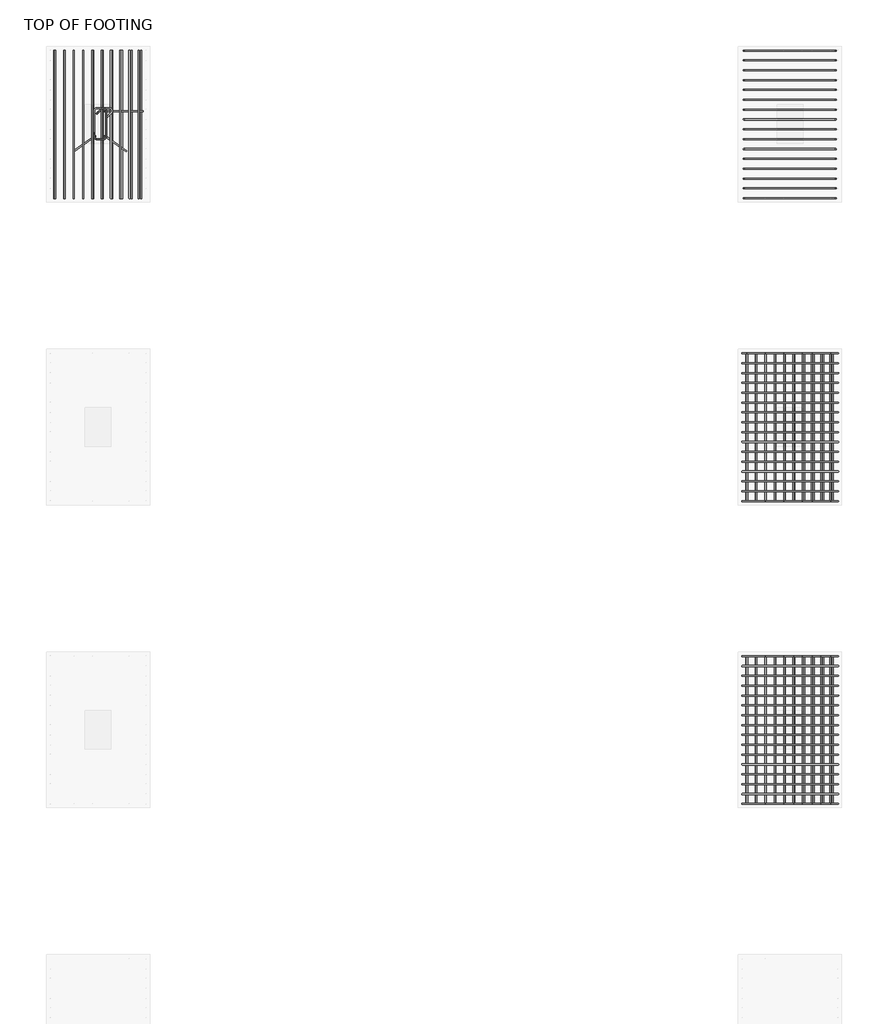
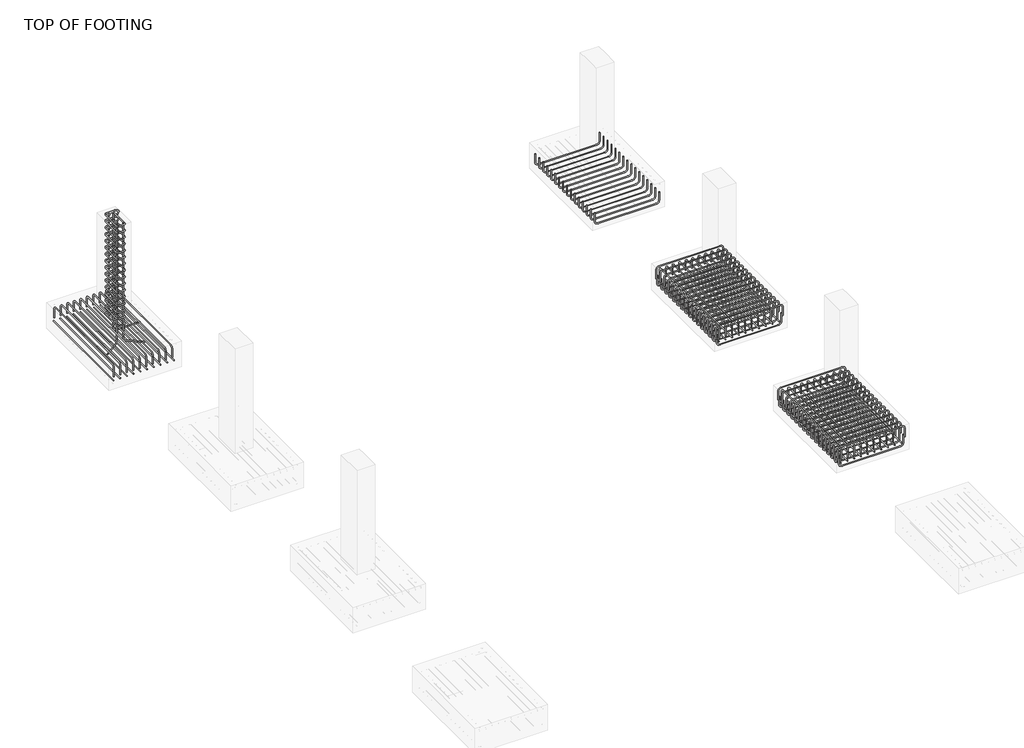
# One storey, part 4 of 8: 15 reinforcing bars.
"""IFC4 building model written with IfcOpenShell, lengths in millimetres."""

from ifc_helpers import new_model, si_unit, point, frame, origin, place, context, project, spatial, polyline, circle_curve, trimmed, segment, composite_curve, source, transform, mapped, element, save
from ifc_brep_helpers import swept_disk

model = new_model("IFC4")

# Units and contexts
model_context = context("Model", 3, world=origin())
ifc_project = project(units=[si_unit("LENGTHUNIT", "METRE", prefix="MILLI")], contexts=[model_context])

# Site, building, storey
site = spatial("IfcSite", under=ifc_project)
building = spatial("IfcBuilding", under=site)
storey = spatial("IfcBuildingStorey", under=building, Name="TOP OF FOOTING", Elevation=-1828.8)

# Reinforcing bars
placement = place(None, origin())
reinforcing_bar_shape = source(origin(), model_context, "Body", "SolidModel", [
    swept_disk(composite_curve([segment(polyline([(-12339.592709, 16632.7008557, -2155.1176129), (-12339.592709, 14912.7008557, -2155.1176129)]), True, "CONTINUOUS")], self_intersect=False), 6.35),
])
element("IfcReinforcingBar", 1, at=placement, inside=storey, context=model_context, shape_type="MappedRepresentation", body=[
    mapped(reinforcing_bar_shape, transform((0.0, 0.0, 0.0), x_axis=(1.0, 0.0, 0.0), y_axis=(0.0, 1.0, 0.0), z_axis=(0.0, 0.0, 1.0))),
    mapped(reinforcing_bar_shape, transform((111.602188, 0.0, 0.0), x_axis=(1.0, 0.0, 0.0), y_axis=(0.0, 1.0, 0.0), z_axis=(0.0, 0.0, 1.0))),
    mapped(reinforcing_bar_shape, transform((223.2043759, 0.0, 0.0), x_axis=(1.0, 0.0, 0.0), y_axis=(0.0, 1.0, 0.0), z_axis=(0.0, 0.0, 1.0))),
    mapped(reinforcing_bar_shape, transform((334.8065639, 0.0, 0.0), x_axis=(1.0, 0.0, 0.0), y_axis=(0.0, 1.0, 0.0), z_axis=(0.0, 0.0, 1.0))),
    mapped(reinforcing_bar_shape, transform((446.4087519, 0.0, 0.0), x_axis=(1.0, 0.0, 0.0), y_axis=(0.0, 1.0, 0.0), z_axis=(0.0, 0.0, 1.0))),
    mapped(reinforcing_bar_shape, transform((558.0109398, 0.0, 0.0), x_axis=(1.0, 0.0, 0.0), y_axis=(0.0, 1.0, 0.0), z_axis=(0.0, 0.0, 1.0))),
    mapped(reinforcing_bar_shape, transform((669.6131278, 0.0, 0.0), x_axis=(1.0, 0.0, 0.0), y_axis=(0.0, 1.0, 0.0), z_axis=(0.0, 0.0, 1.0))),
    mapped(reinforcing_bar_shape, transform((781.2153158, 0.0, 0.0), x_axis=(1.0, 0.0, 0.0), y_axis=(0.0, 1.0, 0.0), z_axis=(0.0, 0.0, 1.0))),
    mapped(reinforcing_bar_shape, transform((892.8175037, 0.0, 0.0), x_axis=(1.0, 0.0, 0.0), y_axis=(0.0, 1.0, 0.0), z_axis=(0.0, 0.0, 1.0))),
    mapped(reinforcing_bar_shape, transform((1004.4196917, 0.0, 0.0), x_axis=(1.0, 0.0, 0.0), y_axis=(0.0, 1.0, 0.0), z_axis=(0.0, 0.0, 1.0))),
])
reinforcing_bar_2_shape = source(origin(), model_context, "Body", "SolidModel", [
    swept_disk(composite_curve([segment(polyline([(-11364.2651981, 16626.3508557, -2094.6521303), (-11364.2651981, 16626.3508557, -1947.3521303)]), True, "CONTINUOUS"), segment(trimmed(circle_curve(frame((-11364.2651981, 16580.0008557, -1947.3521303), z_axis=(1.0, 0.0, 0.0), x_axis=(0.0, 46.349999999998545, 0.0)), 46.35), [point((-11364.2651981, 16626.3508557, -1947.3521303))], [point((-11364.2651981, 16580.0008557, -1901.0021303))], True, "CARTESIAN"), True, "CONTINUOUS"), segment(polyline([(-11364.2651981, 16580.0008557, -1901.0021303), (-11364.2651981, 14965.4008557, -1901.0021303)]), True, "CONTINUOUS"), segment(trimmed(circle_curve(frame((-11364.2651981, 14965.4008557, -1947.3521303), z_axis=(1.0, 0.0, 0.0), x_axis=(0.0, 0.0, 46.34999999999991)), 46.35), [point((-11364.2651981, 14965.4008557, -1901.0021303))], [point((-11364.2651981, 14919.0508557, -1947.3521303))], True, "CARTESIAN"), True, "CONTINUOUS"), segment(polyline([(-11364.2651981, 14919.0508557, -1947.3521303), (-11364.2651981, 14919.0508557, -2094.6521303)]), True, "CONTINUOUS")], self_intersect=False), 6.35),
])
element("IfcReinforcingBar", 2, at=placement, inside=storey, context=model_context, shape_type="MappedRepresentation", body=[
    mapped(reinforcing_bar_2_shape, transform((0.0, 0.0, 0.0), x_axis=(1.0, 0.0, 0.0), y_axis=(0.0, 1.0, 0.0), z_axis=(0.0, 0.0, 1.0))),
    mapped(reinforcing_bar_2_shape, transform((-107.1680233, 0.0, 0.0), x_axis=(1.0, 0.0, 0.0), y_axis=(0.0, 1.0, 0.0), z_axis=(0.0, 0.0, 1.0))),
    mapped(reinforcing_bar_2_shape, transform((-214.3360466, 0.0, 0.0), x_axis=(1.0, 0.0, 0.0), y_axis=(0.0, 1.0, 0.0), z_axis=(0.0, 0.0, 1.0))),
    mapped(reinforcing_bar_2_shape, transform((-321.5040699, 0.0, 0.0), x_axis=(1.0, 0.0, 0.0), y_axis=(0.0, 1.0, 0.0), z_axis=(0.0, 0.0, 1.0))),
    mapped(reinforcing_bar_2_shape, transform((-428.6720932, 0.0, 0.0), x_axis=(1.0, 0.0, 0.0), y_axis=(0.0, 1.0, 0.0), z_axis=(0.0, 0.0, 1.0))),
    mapped(reinforcing_bar_2_shape, transform((-535.8401165, 0.0, 0.0), x_axis=(1.0, 0.0, 0.0), y_axis=(0.0, 1.0, 0.0), z_axis=(0.0, 0.0, 1.0))),
    mapped(reinforcing_bar_2_shape, transform((-643.0081398, 0.0, 0.0), x_axis=(1.0, 0.0, 0.0), y_axis=(0.0, 1.0, 0.0), z_axis=(0.0, 0.0, 1.0))),
    mapped(reinforcing_bar_2_shape, transform((-750.176163, 0.0, 0.0), x_axis=(1.0, 0.0, 0.0), y_axis=(0.0, 1.0, 0.0), z_axis=(0.0, 0.0, 1.0))),
    mapped(reinforcing_bar_2_shape, transform((-857.3441863, 0.0, 0.0), x_axis=(1.0, 0.0, 0.0), y_axis=(0.0, 1.0, 0.0), z_axis=(0.0, 0.0, 1.0))),
    mapped(reinforcing_bar_2_shape, transform((-964.5122096, 0.0, 0.0), x_axis=(1.0, 0.0, 0.0), y_axis=(0.0, 1.0, 0.0), z_axis=(0.0, 0.0, 1.0))),
])
reinforcing_bar_3_shape = source(origin(), model_context, "Body", "SolidModel", [
    swept_disk(composite_curve([segment(polyline([(-11851.3503281, 15894.7413561, -46.35), (-11795.6067652, 15950.484919, -46.35)]), True, "CONTINUOUS"), segment(trimmed(circle_curve(frame((-11773.4389676, 15928.3171214, -46.35), z_axis=(0.0, 0.0, -1.0), x_axis=(-22.167797600000995, 22.167797600000995, 0.0)), 31.35), [point((-11795.6067652, 15950.484919, -46.35))], [point((-11742.0889676, 15928.3171214, -46.35))], True, "CARTESIAN"), True, "CONTINUOUS"), segment(polyline([(-11742.0889676, 15928.3171214, -46.35), (-11742.0889676, 15633.7171214, -46.35)]), True, "CONTINUOUS"), segment(trimmed(circle_curve(frame((-11773.4389676, 15633.7171214, -46.35), z_axis=(0.0, 0.0, -1.0), x_axis=(31.349999999998545, 0.0, 0.0)), 31.35), [point((-11742.0889676, 15633.7171214, -46.35))], [point((-11773.4389676, 15602.3671214, -46.35))], True, "CARTESIAN"), True, "CONTINUOUS"), segment(polyline([(-11773.4389676, 15602.3671214, -46.35), (-11848.385177, 15602.3671214, -46.35)]), True, "CONTINUOUS"), segment(trimmed(circle_curve(frame((-11848.385177, 15633.6973363, -45.2363875), z_axis=(0.0, 0.035521928334481916, -0.9993688971583016), x_axis=(0.0, -31.33021489999919, -1.1136125000000021)), 31.35), [point((-11848.385177, 15602.3671214, -46.35))], [point((-11879.735177, 15633.6973363, -45.2363875))], True, "CARTESIAN"), True, "CONTINUOUS"), segment(polyline([(-11879.735177, 15633.6973363, -45.2363875), (-11879.735177, 15928.3369065, -34.7636125)]), True, "CONTINUOUS"), segment(trimmed(circle_curve(frame((-11848.385177, 15928.3369065, -34.7636125), z_axis=(0.0, 0.035521928334481916, -0.9993688971583016), x_axis=(-31.350000000000364, 0.0, 0.0)), 31.35), [point((-11879.735177, 15928.3369065, -34.7636125))], [point((-11848.385177, 15959.6671214, -33.65))], True, "CARTESIAN"), True, "CONTINUOUS"), segment(polyline([(-11848.385177, 15959.6671214, -33.65), (-11703.785177, 15959.6671214, -33.65)]), True, "CONTINUOUS"), segment(trimmed(circle_curve(frame((-11703.785177, 15928.3171214, -33.65), z_axis=(0.0, 0.0, -1.0), x_axis=(0.0, 31.350000000000364, 0.0)), 31.35), [point((-11703.785177, 15959.6671214, -33.65))], [point((-11681.6173794, 15906.1493238, -33.65))], True, "CARTESIAN"), True, "CONTINUOUS"), segment(polyline([(-11681.6173794, 15906.1493238, -33.65), (-11737.3609424, 15850.4057609, -33.65)]), True, "CONTINUOUS")], self_intersect=False), 6.35),
])
element("IfcReinforcingBar", 3, at=placement, inside=storey, context=model_context, shape_type="MappedRepresentation", body=[
    mapped(reinforcing_bar_3_shape, transform((0.0, 0.0, 0.0), x_axis=(1.0, 0.0, 0.0), y_axis=(0.0, 1.0, 0.0), z_axis=(0.0, 0.0, 1.0))),
    mapped(reinforcing_bar_3_shape, transform((0.0, 0.0, -115.74), x_axis=(1.0, 0.0, 0.0), y_axis=(0.0, 1.0, 0.0), z_axis=(0.0, 0.0, 1.0))),
    mapped(reinforcing_bar_3_shape, transform((0.0, 0.0, -231.48), x_axis=(1.0, 0.0, 0.0), y_axis=(0.0, 1.0, 0.0), z_axis=(0.0, 0.0, 1.0))),
    mapped(reinforcing_bar_3_shape, transform((0.0, 0.0, -347.22), x_axis=(1.0, 0.0, 0.0), y_axis=(0.0, 1.0, 0.0), z_axis=(0.0, 0.0, 1.0))),
    mapped(reinforcing_bar_3_shape, transform((0.0, 0.0, -462.96), x_axis=(1.0, 0.0, 0.0), y_axis=(0.0, 1.0, 0.0), z_axis=(0.0, 0.0, 1.0))),
    mapped(reinforcing_bar_3_shape, transform((0.0, 0.0, -578.7), x_axis=(1.0, 0.0, 0.0), y_axis=(0.0, 1.0, 0.0), z_axis=(0.0, 0.0, 1.0))),
    mapped(reinforcing_bar_3_shape, transform((0.0, 0.0, -694.44), x_axis=(1.0, 0.0, 0.0), y_axis=(0.0, 1.0, 0.0), z_axis=(0.0, 0.0, 1.0))),
    mapped(reinforcing_bar_3_shape, transform((0.0, 0.0, -810.18), x_axis=(1.0, 0.0, 0.0), y_axis=(0.0, 1.0, 0.0), z_axis=(0.0, 0.0, 1.0))),
    mapped(reinforcing_bar_3_shape, transform((0.0, 0.0, -925.92), x_axis=(1.0, 0.0, 0.0), y_axis=(0.0, 1.0, 0.0), z_axis=(0.0, 0.0, 1.0))),
    mapped(reinforcing_bar_3_shape, transform((0.0, 0.0, -1041.66), x_axis=(1.0, 0.0, 0.0), y_axis=(0.0, 1.0, 0.0), z_axis=(0.0, 0.0, 1.0))),
    mapped(reinforcing_bar_3_shape, transform((0.0, 0.0, -1157.4), x_axis=(1.0, 0.0, 0.0), y_axis=(0.0, 1.0, 0.0), z_axis=(0.0, 0.0, 1.0))),
    mapped(reinforcing_bar_3_shape, transform((0.0, 0.0, -1273.14), x_axis=(1.0, 0.0, 0.0), y_axis=(0.0, 1.0, 0.0), z_axis=(0.0, 0.0, 1.0))),
    mapped(reinforcing_bar_3_shape, transform((0.0, 0.0, -1388.88), x_axis=(1.0, 0.0, 0.0), y_axis=(0.0, 1.0, 0.0), z_axis=(0.0, 0.0, 1.0))),
    mapped(reinforcing_bar_3_shape, transform((0.0, 0.0, -1504.62), x_axis=(1.0, 0.0, 0.0), y_axis=(0.0, 1.0, 0.0), z_axis=(0.0, 0.0, 1.0))),
    mapped(reinforcing_bar_3_shape, transform((0.0, 0.0, -1620.36), x_axis=(1.0, 0.0, 0.0), y_axis=(0.0, 1.0, 0.0), z_axis=(0.0, 0.0, 1.0))),
    mapped(reinforcing_bar_3_shape, transform((0.0, 0.0, -1736.1), x_axis=(1.0, 0.0, 0.0), y_axis=(0.0, 1.0, 0.0), z_axis=(0.0, 0.0, 1.0))),
])
element("IfcReinforcingBar", 4, at=placement, inside=storey, context=model_context, shape_type="SolidModel", body=[
    swept_disk(composite_curve([segment(polyline([(-11755.8874017, 15924.2508557, -40.0), (-11755.8874017, 15924.2508557, -2055.5685723)]), True, "CONTINUOUS"), segment(trimmed(circle_curve(frame((-11709.5374017, 15924.2508557, -2055.5685723), z_axis=(0.0, -1.0, 0.0), x_axis=(-46.350000000000364, 0.0, 0.0)), 46.35), [point((-11755.8874017, 15924.2508557, -2055.5685723))], [point((-11709.5374017, 15924.2508557, -2101.9185723))], True, "CARTESIAN"), True, "CONTINUOUS"), segment(polyline([(-11709.5374017, 15924.2508557, -2101.9185723), (-11315.6661764, 15924.2508557, -2101.9185723)]), True, "CONTINUOUS")], self_intersect=False), 6.35),
])
element("IfcReinforcingBar", 5, at=placement, inside=storey, context=model_context, shape_type="SolidModel", body=[
    swept_disk(composite_curve([segment(polyline([(-11755.8874017, 15637.7833871, -40.0), (-11755.8874017, 15637.7833871, -2055.5685723)]), True, "CONTINUOUS"), segment(trimmed(circle_curve(frame((-11717.9197045, 15611.1981193, -2055.5685723), z_axis=(-0.5735764363510459, -0.819152044288992, 0.0), x_axis=(-37.96769719999975, 26.58526780000102, 0.0)), 46.35), [point((-11755.8874017, 15637.7833871, -2055.5685723))], [point((-11717.9197045, 15611.1981193, -2101.9185723))], True, "CARTESIAN"), True, "CONTINUOUS"), segment(polyline([(-11717.9197045, 15611.1981193, -2101.9185723), (-11506.0932621, 15462.8756476, -2101.9185723)]), True, "CONTINUOUS")], self_intersect=False), 6.35),
])
element("IfcReinforcingBar", 6, at=placement, inside=storey, context=model_context, shape_type="SolidModel", body=[
    swept_disk(composite_curve([segment(polyline([(-11865.9367429, 15637.7833871, -40.0), (-11865.9367429, 15637.7833871, -2055.5685723)]), True, "CONTINUOUS"), segment(trimmed(circle_curve(frame((-11903.9044402, 15611.1981193, -2055.5685723), z_axis=(-0.5735764363510459, 0.819152044288992, 0.0), x_axis=(37.96769730000051, 26.58526780000102, 0.0)), 46.35), [point((-11865.9367429, 15637.7833871, -2055.5685723))], [point((-11903.9044402, 15611.1981193, -2101.9185723))], True, "CARTESIAN"), True, "CONTINUOUS"), segment(polyline([(-11903.9044402, 15611.1981193, -2101.9185723), (-12115.7308826, 15462.8756476, -2101.9185723)]), True, "CONTINUOUS")], self_intersect=False), 6.35),
])
reinforcing_bar_4_shape = source(origin(), model_context, "Body", "SolidModel", [
    swept_disk(composite_curve([segment(polyline([(-3301.5220197, 16626.3508557, -2021.4413313), (-3301.5220197, 16626.3508557, -2168.7413313)]), True, "CONTINUOUS"), segment(trimmed(circle_curve(frame((-3347.8720197, 16626.3508557, -2168.7413313), z_axis=(0.0, 1.0, 0.0), x_axis=(46.34999999999991, 0.0, 0.0)), 46.35), [point((-3301.5220197, 16626.3508557, -2168.7413313))], [point((-3347.8720197, 16626.3508557, -2215.0913313))], True, "CARTESIAN"), True, "CONTINUOUS"), segment(polyline([(-3347.8720197, 16626.3508557, -2215.0913313), (-4320.167031, 16626.3508557, -2215.0913313)]), True, "CONTINUOUS"), segment(trimmed(circle_curve(frame((-4320.167031, 16626.3508557, -2168.7413313), z_axis=(0.0, 1.0, 0.0), x_axis=(0.0, 0.0, -46.34999999999991)), 46.35), [point((-4320.167031, 16626.3508557, -2215.0913313))], [point((-4366.517031, 16626.3508557, -2168.7413313))], True, "CARTESIAN"), True, "CONTINUOUS"), segment(polyline([(-4366.517031, 16626.3508557, -2168.7413313), (-4366.517031, 16626.3508557, -2021.4413313)]), True, "CONTINUOUS")], self_intersect=False), 6.35),
])
element("IfcReinforcingBar", 7, at=placement, inside=storey, context=model_context, shape_type="MappedRepresentation", body=[
    mapped(reinforcing_bar_4_shape, transform((0.0, 0.0, 0.0), x_axis=(1.0, 0.0, 0.0), y_axis=(0.0, 1.0, 0.0), z_axis=(0.0, 0.0, 1.0))),
    mapped(reinforcing_bar_4_shape, transform((0.0, -113.82, 0.0), x_axis=(1.0, 0.0, 0.0), y_axis=(0.0, 1.0, 0.0), z_axis=(0.0, 0.0, 1.0))),
    mapped(reinforcing_bar_4_shape, transform((0.0, -227.64, 0.0), x_axis=(1.0, 0.0, 0.0), y_axis=(0.0, 1.0, 0.0), z_axis=(0.0, 0.0, 1.0))),
    mapped(reinforcing_bar_4_shape, transform((0.0, -341.46, 0.0), x_axis=(1.0, 0.0, 0.0), y_axis=(0.0, 1.0, 0.0), z_axis=(0.0, 0.0, 1.0))),
    mapped(reinforcing_bar_4_shape, transform((0.0, -455.28, 0.0), x_axis=(1.0, 0.0, 0.0), y_axis=(0.0, 1.0, 0.0), z_axis=(0.0, 0.0, 1.0))),
    mapped(reinforcing_bar_4_shape, transform((0.0, -569.1, 0.0), x_axis=(1.0, 0.0, 0.0), y_axis=(0.0, 1.0, 0.0), z_axis=(0.0, 0.0, 1.0))),
    mapped(reinforcing_bar_4_shape, transform((0.0, -682.92, 0.0), x_axis=(1.0, 0.0, 0.0), y_axis=(0.0, 1.0, 0.0), z_axis=(0.0, 0.0, 1.0))),
    mapped(reinforcing_bar_4_shape, transform((0.0, -796.74, 0.0), x_axis=(1.0, 0.0, 0.0), y_axis=(0.0, 1.0, 0.0), z_axis=(0.0, 0.0, 1.0))),
    mapped(reinforcing_bar_4_shape, transform((0.0, -910.56, 0.0), x_axis=(1.0, 0.0, 0.0), y_axis=(0.0, 1.0, 0.0), z_axis=(0.0, 0.0, 1.0))),
    mapped(reinforcing_bar_4_shape, transform((0.0, -1024.38, 0.0), x_axis=(1.0, 0.0, 0.0), y_axis=(0.0, 1.0, 0.0), z_axis=(0.0, 0.0, 1.0))),
    mapped(reinforcing_bar_4_shape, transform((0.0, -1138.2, 0.0), x_axis=(1.0, 0.0, 0.0), y_axis=(0.0, 1.0, 0.0), z_axis=(0.0, 0.0, 1.0))),
    mapped(reinforcing_bar_4_shape, transform((0.0, -1252.02, 0.0), x_axis=(1.0, 0.0, 0.0), y_axis=(0.0, 1.0, 0.0), z_axis=(0.0, 0.0, 1.0))),
    mapped(reinforcing_bar_4_shape, transform((0.0, -1365.84, 0.0), x_axis=(1.0, 0.0, 0.0), y_axis=(0.0, 1.0, 0.0), z_axis=(0.0, 0.0, 1.0))),
    mapped(reinforcing_bar_4_shape, transform((0.0, -1479.66, 0.0), x_axis=(1.0, 0.0, 0.0), y_axis=(0.0, 1.0, 0.0), z_axis=(0.0, 0.0, 1.0))),
    mapped(reinforcing_bar_4_shape, transform((0.0, -1593.48, 0.0), x_axis=(1.0, 0.0, 0.0), y_axis=(0.0, 1.0, 0.0), z_axis=(0.0, 0.0, 1.0))),
    mapped(reinforcing_bar_4_shape, transform((0.0, -1707.3, 0.0), x_axis=(1.0, 0.0, 0.0), y_axis=(0.0, 1.0, 0.0), z_axis=(0.0, 0.0, 1.0))),
])
reinforcing_bar_5_shape = source(origin(), model_context, "Body", "SolidModel", [
    swept_disk(composite_curve([segment(polyline([(-3301.5220197, 13126.3508557, -2021.4413313), (-3301.5220197, 13126.3508557, -2168.7413313)]), True, "CONTINUOUS"), segment(trimmed(circle_curve(frame((-3347.8720197, 13126.3508557, -2168.7413313), z_axis=(0.0, 1.0, 0.0), x_axis=(46.34999999999991, 0.0, 0.0)), 46.35), [point((-3301.5220197, 13126.3508557, -2168.7413313))], [point((-3347.8720197, 13126.3508557, -2215.0913313))], True, "CARTESIAN"), True, "CONTINUOUS"), segment(polyline([(-3347.8720197, 13126.3508557, -2215.0913313), (-4320.167031, 13126.3508557, -2215.0913313)]), True, "CONTINUOUS"), segment(trimmed(circle_curve(frame((-4320.167031, 13126.3508557, -2168.7413313), z_axis=(0.0, 1.0, 0.0), x_axis=(0.0, 0.0, -46.34999999999991)), 46.35), [point((-4320.167031, 13126.3508557, -2215.0913313))], [point((-4366.517031, 13126.3508557, -2168.7413313))], True, "CARTESIAN"), True, "CONTINUOUS"), segment(polyline([(-4366.517031, 13126.3508557, -2168.7413313), (-4366.517031, 13126.3508557, -2021.4413313)]), True, "CONTINUOUS")], self_intersect=False), 6.35),
])
element("IfcReinforcingBar", 8, at=placement, inside=storey, context=model_context, shape_type="MappedRepresentation", body=[
    mapped(reinforcing_bar_5_shape, transform((0.0, 0.0, 0.0), x_axis=(1.0, 0.0, 0.0), y_axis=(0.0, 1.0, 0.0), z_axis=(0.0, 0.0, 1.0))),
    mapped(reinforcing_bar_5_shape, transform((0.0, -113.82, 0.0), x_axis=(1.0, 0.0, 0.0), y_axis=(0.0, 1.0, 0.0), z_axis=(0.0, 0.0, 1.0))),
    mapped(reinforcing_bar_5_shape, transform((0.0, -227.64, 0.0), x_axis=(1.0, 0.0, 0.0), y_axis=(0.0, 1.0, 0.0), z_axis=(0.0, 0.0, 1.0))),
    mapped(reinforcing_bar_5_shape, transform((0.0, -341.46, 0.0), x_axis=(1.0, 0.0, 0.0), y_axis=(0.0, 1.0, 0.0), z_axis=(0.0, 0.0, 1.0))),
    mapped(reinforcing_bar_5_shape, transform((0.0, -455.28, 0.0), x_axis=(1.0, 0.0, 0.0), y_axis=(0.0, 1.0, 0.0), z_axis=(0.0, 0.0, 1.0))),
    mapped(reinforcing_bar_5_shape, transform((0.0, -569.1, 0.0), x_axis=(1.0, 0.0, 0.0), y_axis=(0.0, 1.0, 0.0), z_axis=(0.0, 0.0, 1.0))),
    mapped(reinforcing_bar_5_shape, transform((0.0, -682.92, 0.0), x_axis=(1.0, 0.0, 0.0), y_axis=(0.0, 1.0, 0.0), z_axis=(0.0, 0.0, 1.0))),
    mapped(reinforcing_bar_5_shape, transform((0.0, -796.74, 0.0), x_axis=(1.0, 0.0, 0.0), y_axis=(0.0, 1.0, 0.0), z_axis=(0.0, 0.0, 1.0))),
    mapped(reinforcing_bar_5_shape, transform((0.0, -910.56, 0.0), x_axis=(1.0, 0.0, 0.0), y_axis=(0.0, 1.0, 0.0), z_axis=(0.0, 0.0, 1.0))),
    mapped(reinforcing_bar_5_shape, transform((0.0, -1024.38, 0.0), x_axis=(1.0, 0.0, 0.0), y_axis=(0.0, 1.0, 0.0), z_axis=(0.0, 0.0, 1.0))),
    mapped(reinforcing_bar_5_shape, transform((0.0, -1138.2, 0.0), x_axis=(1.0, 0.0, 0.0), y_axis=(0.0, 1.0, 0.0), z_axis=(0.0, 0.0, 1.0))),
    mapped(reinforcing_bar_5_shape, transform((0.0, -1252.02, 0.0), x_axis=(1.0, 0.0, 0.0), y_axis=(0.0, 1.0, 0.0), z_axis=(0.0, 0.0, 1.0))),
    mapped(reinforcing_bar_5_shape, transform((0.0, -1365.84, 0.0), x_axis=(1.0, 0.0, 0.0), y_axis=(0.0, 1.0, 0.0), z_axis=(0.0, 0.0, 1.0))),
    mapped(reinforcing_bar_5_shape, transform((0.0, -1479.66, 0.0), x_axis=(1.0, 0.0, 0.0), y_axis=(0.0, 1.0, 0.0), z_axis=(0.0, 0.0, 1.0))),
    mapped(reinforcing_bar_5_shape, transform((0.0, -1593.48, 0.0), x_axis=(1.0, 0.0, 0.0), y_axis=(0.0, 1.0, 0.0), z_axis=(0.0, 0.0, 1.0))),
    mapped(reinforcing_bar_5_shape, transform((0.0, -1707.3, 0.0), x_axis=(1.0, 0.0, 0.0), y_axis=(0.0, 1.0, 0.0), z_axis=(0.0, 0.0, 1.0))),
])
reinforcing_bar_6_shape = source(origin(), model_context, "Body", "SolidModel", [
    swept_disk(composite_curve([segment(polyline([(-4384.3374017, 13126.3508557, -2068.8), (-4384.3374017, 13126.3508557, -1921.5)]), True, "CONTINUOUS"), segment(trimmed(circle_curve(frame((-4337.9874017, 13126.3508557, -1921.5), z_axis=(0.0, 1.0, 0.0), x_axis=(-46.349999999999454, 0.0, 0.0)), 46.35), [point((-4384.3374017, 13126.3508557, -1921.5))], [point((-4337.9874017, 13126.3508557, -1875.15))], True, "CARTESIAN"), True, "CONTINUOUS"), segment(polyline([(-4337.9874017, 13126.3508557, -1875.15), (-3323.3874017, 13126.3508557, -1875.15)]), True, "CONTINUOUS"), segment(trimmed(circle_curve(frame((-3323.3874017, 13126.3508557, -1921.5), z_axis=(0.0, 1.0, 0.0), x_axis=(0.0, 0.0, 46.34999999999991)), 46.35), [point((-3323.3874017, 13126.3508557, -1875.15))], [point((-3277.0374017, 13126.3508557, -1921.5))], True, "CARTESIAN"), True, "CONTINUOUS"), segment(polyline([(-3277.0374017, 13126.3508557, -1921.5), (-3277.0374017, 13126.3508557, -2068.8)]), True, "CONTINUOUS")], self_intersect=False), 6.35),
])
element("IfcReinforcingBar", 9, at=placement, inside=storey, context=model_context, shape_type="MappedRepresentation", body=[
    mapped(reinforcing_bar_6_shape, transform((0.0, 0.0, 0.0), x_axis=(1.0, 0.0, 0.0), y_axis=(0.0, 1.0, 0.0), z_axis=(0.0, 0.0, 1.0))),
    mapped(reinforcing_bar_6_shape, transform((0.0, -113.82, 0.0), x_axis=(1.0, 0.0, 0.0), y_axis=(0.0, 1.0, 0.0), z_axis=(0.0, 0.0, 1.0))),
    mapped(reinforcing_bar_6_shape, transform((0.0, -227.64, 0.0), x_axis=(1.0, 0.0, 0.0), y_axis=(0.0, 1.0, 0.0), z_axis=(0.0, 0.0, 1.0))),
    mapped(reinforcing_bar_6_shape, transform((0.0, -341.46, 0.0), x_axis=(1.0, 0.0, 0.0), y_axis=(0.0, 1.0, 0.0), z_axis=(0.0, 0.0, 1.0))),
    mapped(reinforcing_bar_6_shape, transform((0.0, -455.28, 0.0), x_axis=(1.0, 0.0, 0.0), y_axis=(0.0, 1.0, 0.0), z_axis=(0.0, 0.0, 1.0))),
    mapped(reinforcing_bar_6_shape, transform((0.0, -569.1, 0.0), x_axis=(1.0, 0.0, 0.0), y_axis=(0.0, 1.0, 0.0), z_axis=(0.0, 0.0, 1.0))),
    mapped(reinforcing_bar_6_shape, transform((0.0, -682.92, 0.0), x_axis=(1.0, 0.0, 0.0), y_axis=(0.0, 1.0, 0.0), z_axis=(0.0, 0.0, 1.0))),
    mapped(reinforcing_bar_6_shape, transform((0.0, -796.74, 0.0), x_axis=(1.0, 0.0, 0.0), y_axis=(0.0, 1.0, 0.0), z_axis=(0.0, 0.0, 1.0))),
    mapped(reinforcing_bar_6_shape, transform((0.0, -910.56, 0.0), x_axis=(1.0, 0.0, 0.0), y_axis=(0.0, 1.0, 0.0), z_axis=(0.0, 0.0, 1.0))),
    mapped(reinforcing_bar_6_shape, transform((0.0, -1024.38, 0.0), x_axis=(1.0, 0.0, 0.0), y_axis=(0.0, 1.0, 0.0), z_axis=(0.0, 0.0, 1.0))),
    mapped(reinforcing_bar_6_shape, transform((0.0, -1138.2, 0.0), x_axis=(1.0, 0.0, 0.0), y_axis=(0.0, 1.0, 0.0), z_axis=(0.0, 0.0, 1.0))),
    mapped(reinforcing_bar_6_shape, transform((0.0, -1252.02, 0.0), x_axis=(1.0, 0.0, 0.0), y_axis=(0.0, 1.0, 0.0), z_axis=(0.0, 0.0, 1.0))),
    mapped(reinforcing_bar_6_shape, transform((0.0, -1365.84, 0.0), x_axis=(1.0, 0.0, 0.0), y_axis=(0.0, 1.0, 0.0), z_axis=(0.0, 0.0, 1.0))),
    mapped(reinforcing_bar_6_shape, transform((0.0, -1479.66, 0.0), x_axis=(1.0, 0.0, 0.0), y_axis=(0.0, 1.0, 0.0), z_axis=(0.0, 0.0, 1.0))),
    mapped(reinforcing_bar_6_shape, transform((0.0, -1593.48, 0.0), x_axis=(1.0, 0.0, 0.0), y_axis=(0.0, 1.0, 0.0), z_axis=(0.0, 0.0, 1.0))),
    mapped(reinforcing_bar_6_shape, transform((0.0, -1707.3, 0.0), x_axis=(1.0, 0.0, 0.0), y_axis=(0.0, 1.0, 0.0), z_axis=(0.0, 0.0, 1.0))),
])
reinforcing_bar_7_shape = source(origin(), model_context, "Body", "SolidModel", [
    swept_disk(composite_curve([segment(polyline([(-4339.592709, 13132.7008557, -2155.1176129), (-4339.592709, 11412.7008557, -2155.1176129)]), True, "CONTINUOUS")], self_intersect=False), 6.35),
])
element("IfcReinforcingBar", 10, at=placement, inside=storey, context=model_context, shape_type="MappedRepresentation", body=[
    mapped(reinforcing_bar_7_shape, transform((0.0, 0.0, 0.0), x_axis=(1.0, 0.0, 0.0), y_axis=(0.0, 1.0, 0.0), z_axis=(0.0, 0.0, 1.0))),
    mapped(reinforcing_bar_7_shape, transform((111.602188, 0.0, 0.0), x_axis=(1.0, 0.0, 0.0), y_axis=(0.0, 1.0, 0.0), z_axis=(0.0, 0.0, 1.0))),
    mapped(reinforcing_bar_7_shape, transform((223.2043759, 0.0, 0.0), x_axis=(1.0, 0.0, 0.0), y_axis=(0.0, 1.0, 0.0), z_axis=(0.0, 0.0, 1.0))),
    mapped(reinforcing_bar_7_shape, transform((334.8065639, 0.0, 0.0), x_axis=(1.0, 0.0, 0.0), y_axis=(0.0, 1.0, 0.0), z_axis=(0.0, 0.0, 1.0))),
    mapped(reinforcing_bar_7_shape, transform((446.4087519, 0.0, 0.0), x_axis=(1.0, 0.0, 0.0), y_axis=(0.0, 1.0, 0.0), z_axis=(0.0, 0.0, 1.0))),
    mapped(reinforcing_bar_7_shape, transform((558.0109398, 0.0, 0.0), x_axis=(1.0, 0.0, 0.0), y_axis=(0.0, 1.0, 0.0), z_axis=(0.0, 0.0, 1.0))),
    mapped(reinforcing_bar_7_shape, transform((669.6131278, 0.0, 0.0), x_axis=(1.0, 0.0, 0.0), y_axis=(0.0, 1.0, 0.0), z_axis=(0.0, 0.0, 1.0))),
    mapped(reinforcing_bar_7_shape, transform((781.2153158, 0.0, 0.0), x_axis=(1.0, 0.0, 0.0), y_axis=(0.0, 1.0, 0.0), z_axis=(0.0, 0.0, 1.0))),
    mapped(reinforcing_bar_7_shape, transform((892.8175037, 0.0, 0.0), x_axis=(1.0, 0.0, 0.0), y_axis=(0.0, 1.0, 0.0), z_axis=(0.0, 0.0, 1.0))),
    mapped(reinforcing_bar_7_shape, transform((1004.4196917, 0.0, 0.0), x_axis=(1.0, 0.0, 0.0), y_axis=(0.0, 1.0, 0.0), z_axis=(0.0, 0.0, 1.0))),
])
reinforcing_bar_8_shape = source(origin(), model_context, "Body", "SolidModel", [
    swept_disk(composite_curve([segment(polyline([(-3364.2651981, 13126.3508557, -2094.6521303), (-3364.2651981, 13126.3508557, -1947.3521303)]), True, "CONTINUOUS"), segment(trimmed(circle_curve(frame((-3364.2651981, 13080.0008557, -1947.3521303), z_axis=(1.0, 0.0, 0.0), x_axis=(0.0, 46.350000000000364, 0.0)), 46.35), [point((-3364.2651981, 13126.3508557, -1947.3521303))], [point((-3364.2651981, 13080.0008557, -1901.0021303))], True, "CARTESIAN"), True, "CONTINUOUS"), segment(polyline([(-3364.2651981, 13080.0008557, -1901.0021303), (-3364.2651981, 11465.4008557, -1901.0021303)]), True, "CONTINUOUS"), segment(trimmed(circle_curve(frame((-3364.2651981, 11465.4008557, -1947.3521303), z_axis=(1.0, 0.0, 0.0), x_axis=(0.0, 0.0, 46.34999999999991)), 46.35), [point((-3364.2651981, 11465.4008557, -1901.0021303))], [point((-3364.2651981, 11419.0508557, -1947.3521303))], True, "CARTESIAN"), True, "CONTINUOUS"), segment(polyline([(-3364.2651981, 11419.0508557, -1947.3521303), (-3364.2651981, 11419.0508557, -2094.6521303)]), True, "CONTINUOUS")], self_intersect=False), 6.35),
])
element("IfcReinforcingBar", 11, at=placement, inside=storey, context=model_context, shape_type="MappedRepresentation", body=[
    mapped(reinforcing_bar_8_shape, transform((0.0, 0.0, 0.0), x_axis=(1.0, 0.0, 0.0), y_axis=(0.0, 1.0, 0.0), z_axis=(0.0, 0.0, 1.0))),
    mapped(reinforcing_bar_8_shape, transform((-107.1680233, 0.0, 0.0), x_axis=(1.0, 0.0, 0.0), y_axis=(0.0, 1.0, 0.0), z_axis=(0.0, 0.0, 1.0))),
    mapped(reinforcing_bar_8_shape, transform((-214.3360466, 0.0, 0.0), x_axis=(1.0, 0.0, 0.0), y_axis=(0.0, 1.0, 0.0), z_axis=(0.0, 0.0, 1.0))),
    mapped(reinforcing_bar_8_shape, transform((-321.5040699, 0.0, 0.0), x_axis=(1.0, 0.0, 0.0), y_axis=(0.0, 1.0, 0.0), z_axis=(0.0, 0.0, 1.0))),
    mapped(reinforcing_bar_8_shape, transform((-428.6720932, 0.0, 0.0), x_axis=(1.0, 0.0, 0.0), y_axis=(0.0, 1.0, 0.0), z_axis=(0.0, 0.0, 1.0))),
    mapped(reinforcing_bar_8_shape, transform((-535.8401165, 0.0, 0.0), x_axis=(1.0, 0.0, 0.0), y_axis=(0.0, 1.0, 0.0), z_axis=(0.0, 0.0, 1.0))),
    mapped(reinforcing_bar_8_shape, transform((-643.0081398, 0.0, 0.0), x_axis=(1.0, 0.0, 0.0), y_axis=(0.0, 1.0, 0.0), z_axis=(0.0, 0.0, 1.0))),
    mapped(reinforcing_bar_8_shape, transform((-750.176163, 0.0, 0.0), x_axis=(1.0, 0.0, 0.0), y_axis=(0.0, 1.0, 0.0), z_axis=(0.0, 0.0, 1.0))),
    mapped(reinforcing_bar_8_shape, transform((-857.3441863, 0.0, 0.0), x_axis=(1.0, 0.0, 0.0), y_axis=(0.0, 1.0, 0.0), z_axis=(0.0, 0.0, 1.0))),
    mapped(reinforcing_bar_8_shape, transform((-964.5122096, 0.0, 0.0), x_axis=(1.0, 0.0, 0.0), y_axis=(0.0, 1.0, 0.0), z_axis=(0.0, 0.0, 1.0))),
])
reinforcing_bar_9_shape = source(origin(), model_context, "Body", "SolidModel", [
    swept_disk(composite_curve([segment(polyline([(-3301.5220197, 9626.3508557, -2021.4413313), (-3301.5220197, 9626.3508557, -2168.7413313)]), True, "CONTINUOUS"), segment(trimmed(circle_curve(frame((-3347.8720197, 9626.3508557, -2168.7413313), z_axis=(0.0, 1.0, 0.0), x_axis=(46.34999999999991, 0.0, 0.0)), 46.35), [point((-3301.5220197, 9626.3508557, -2168.7413313))], [point((-3347.8720197, 9626.3508557, -2215.0913313))], True, "CARTESIAN"), True, "CONTINUOUS"), segment(polyline([(-3347.8720197, 9626.3508557, -2215.0913313), (-4320.167031, 9626.3508557, -2215.0913313)]), True, "CONTINUOUS"), segment(trimmed(circle_curve(frame((-4320.167031, 9626.3508557, -2168.7413313), z_axis=(0.0, 1.0, 0.0), x_axis=(0.0, 0.0, -46.34999999999991)), 46.35), [point((-4320.167031, 9626.3508557, -2215.0913313))], [point((-4366.517031, 9626.3508557, -2168.7413313))], True, "CARTESIAN"), True, "CONTINUOUS"), segment(polyline([(-4366.517031, 9626.3508557, -2168.7413313), (-4366.517031, 9626.3508557, -2021.4413313)]), True, "CONTINUOUS")], self_intersect=False), 6.35),
])
element("IfcReinforcingBar", 12, at=placement, inside=storey, context=model_context, shape_type="MappedRepresentation", body=[
    mapped(reinforcing_bar_9_shape, transform((0.0, 0.0, 0.0), x_axis=(1.0, 0.0, 0.0), y_axis=(0.0, 1.0, 0.0), z_axis=(0.0, 0.0, 1.0))),
    mapped(reinforcing_bar_9_shape, transform((0.0, -113.82, 0.0), x_axis=(1.0, 0.0, 0.0), y_axis=(0.0, 1.0, 0.0), z_axis=(0.0, 0.0, 1.0))),
    mapped(reinforcing_bar_9_shape, transform((0.0, -227.64, 0.0), x_axis=(1.0, 0.0, 0.0), y_axis=(0.0, 1.0, 0.0), z_axis=(0.0, 0.0, 1.0))),
    mapped(reinforcing_bar_9_shape, transform((0.0, -341.46, 0.0), x_axis=(1.0, 0.0, 0.0), y_axis=(0.0, 1.0, 0.0), z_axis=(0.0, 0.0, 1.0))),
    mapped(reinforcing_bar_9_shape, transform((0.0, -455.28, 0.0), x_axis=(1.0, 0.0, 0.0), y_axis=(0.0, 1.0, 0.0), z_axis=(0.0, 0.0, 1.0))),
    mapped(reinforcing_bar_9_shape, transform((0.0, -569.1, 0.0), x_axis=(1.0, 0.0, 0.0), y_axis=(0.0, 1.0, 0.0), z_axis=(0.0, 0.0, 1.0))),
    mapped(reinforcing_bar_9_shape, transform((0.0, -682.92, 0.0), x_axis=(1.0, 0.0, 0.0), y_axis=(0.0, 1.0, 0.0), z_axis=(0.0, 0.0, 1.0))),
    mapped(reinforcing_bar_9_shape, transform((0.0, -796.74, 0.0), x_axis=(1.0, 0.0, 0.0), y_axis=(0.0, 1.0, 0.0), z_axis=(0.0, 0.0, 1.0))),
    mapped(reinforcing_bar_9_shape, transform((0.0, -910.56, 0.0), x_axis=(1.0, 0.0, 0.0), y_axis=(0.0, 1.0, 0.0), z_axis=(0.0, 0.0, 1.0))),
    mapped(reinforcing_bar_9_shape, transform((0.0, -1024.38, 0.0), x_axis=(1.0, 0.0, 0.0), y_axis=(0.0, 1.0, 0.0), z_axis=(0.0, 0.0, 1.0))),
    mapped(reinforcing_bar_9_shape, transform((0.0, -1138.2, 0.0), x_axis=(1.0, 0.0, 0.0), y_axis=(0.0, 1.0, 0.0), z_axis=(0.0, 0.0, 1.0))),
    mapped(reinforcing_bar_9_shape, transform((0.0, -1252.02, 0.0), x_axis=(1.0, 0.0, 0.0), y_axis=(0.0, 1.0, 0.0), z_axis=(0.0, 0.0, 1.0))),
    mapped(reinforcing_bar_9_shape, transform((0.0, -1365.84, 0.0), x_axis=(1.0, 0.0, 0.0), y_axis=(0.0, 1.0, 0.0), z_axis=(0.0, 0.0, 1.0))),
    mapped(reinforcing_bar_9_shape, transform((0.0, -1479.66, 0.0), x_axis=(1.0, 0.0, 0.0), y_axis=(0.0, 1.0, 0.0), z_axis=(0.0, 0.0, 1.0))),
    mapped(reinforcing_bar_9_shape, transform((0.0, -1593.48, 0.0), x_axis=(1.0, 0.0, 0.0), y_axis=(0.0, 1.0, 0.0), z_axis=(0.0, 0.0, 1.0))),
    mapped(reinforcing_bar_9_shape, transform((0.0, -1707.3, 0.0), x_axis=(1.0, 0.0, 0.0), y_axis=(0.0, 1.0, 0.0), z_axis=(0.0, 0.0, 1.0))),
])
reinforcing_bar_10_shape = source(origin(), model_context, "Body", "SolidModel", [
    swept_disk(composite_curve([segment(polyline([(-4384.3374017, 9626.3508557, -2068.8), (-4384.3374017, 9626.3508557, -1921.5)]), True, "CONTINUOUS"), segment(trimmed(circle_curve(frame((-4337.9874017, 9626.3508557, -1921.5), z_axis=(0.0, 1.0, 0.0), x_axis=(-46.349999999999454, 0.0, 0.0)), 46.35), [point((-4384.3374017, 9626.3508557, -1921.5))], [point((-4337.9874017, 9626.3508557, -1875.15))], True, "CARTESIAN"), True, "CONTINUOUS"), segment(polyline([(-4337.9874017, 9626.3508557, -1875.15), (-3323.3874017, 9626.3508557, -1875.15)]), True, "CONTINUOUS"), segment(trimmed(circle_curve(frame((-3323.3874017, 9626.3508557, -1921.5), z_axis=(0.0, 1.0, 0.0), x_axis=(0.0, 0.0, 46.34999999999991)), 46.35), [point((-3323.3874017, 9626.3508557, -1875.15))], [point((-3277.0374017, 9626.3508557, -1921.5))], True, "CARTESIAN"), True, "CONTINUOUS"), segment(polyline([(-3277.0374017, 9626.3508557, -1921.5), (-3277.0374017, 9626.3508557, -2068.8)]), True, "CONTINUOUS")], self_intersect=False), 6.35),
])
element("IfcReinforcingBar", 13, at=placement, inside=storey, context=model_context, shape_type="MappedRepresentation", body=[
    mapped(reinforcing_bar_10_shape, transform((0.0, 0.0, 0.0), x_axis=(1.0, 0.0, 0.0), y_axis=(0.0, 1.0, 0.0), z_axis=(0.0, 0.0, 1.0))),
    mapped(reinforcing_bar_10_shape, transform((0.0, -113.82, 0.0), x_axis=(1.0, 0.0, 0.0), y_axis=(0.0, 1.0, 0.0), z_axis=(0.0, 0.0, 1.0))),
    mapped(reinforcing_bar_10_shape, transform((0.0, -227.64, 0.0), x_axis=(1.0, 0.0, 0.0), y_axis=(0.0, 1.0, 0.0), z_axis=(0.0, 0.0, 1.0))),
    mapped(reinforcing_bar_10_shape, transform((0.0, -341.46, 0.0), x_axis=(1.0, 0.0, 0.0), y_axis=(0.0, 1.0, 0.0), z_axis=(0.0, 0.0, 1.0))),
    mapped(reinforcing_bar_10_shape, transform((0.0, -455.28, 0.0), x_axis=(1.0, 0.0, 0.0), y_axis=(0.0, 1.0, 0.0), z_axis=(0.0, 0.0, 1.0))),
    mapped(reinforcing_bar_10_shape, transform((0.0, -569.1, 0.0), x_axis=(1.0, 0.0, 0.0), y_axis=(0.0, 1.0, 0.0), z_axis=(0.0, 0.0, 1.0))),
    mapped(reinforcing_bar_10_shape, transform((0.0, -682.92, 0.0), x_axis=(1.0, 0.0, 0.0), y_axis=(0.0, 1.0, 0.0), z_axis=(0.0, 0.0, 1.0))),
    mapped(reinforcing_bar_10_shape, transform((0.0, -796.74, 0.0), x_axis=(1.0, 0.0, 0.0), y_axis=(0.0, 1.0, 0.0), z_axis=(0.0, 0.0, 1.0))),
    mapped(reinforcing_bar_10_shape, transform((0.0, -910.56, 0.0), x_axis=(1.0, 0.0, 0.0), y_axis=(0.0, 1.0, 0.0), z_axis=(0.0, 0.0, 1.0))),
    mapped(reinforcing_bar_10_shape, transform((0.0, -1024.38, 0.0), x_axis=(1.0, 0.0, 0.0), y_axis=(0.0, 1.0, 0.0), z_axis=(0.0, 0.0, 1.0))),
    mapped(reinforcing_bar_10_shape, transform((0.0, -1138.2, 0.0), x_axis=(1.0, 0.0, 0.0), y_axis=(0.0, 1.0, 0.0), z_axis=(0.0, 0.0, 1.0))),
    mapped(reinforcing_bar_10_shape, transform((0.0, -1252.02, 0.0), x_axis=(1.0, 0.0, 0.0), y_axis=(0.0, 1.0, 0.0), z_axis=(0.0, 0.0, 1.0))),
    mapped(reinforcing_bar_10_shape, transform((0.0, -1365.84, 0.0), x_axis=(1.0, 0.0, 0.0), y_axis=(0.0, 1.0, 0.0), z_axis=(0.0, 0.0, 1.0))),
    mapped(reinforcing_bar_10_shape, transform((0.0, -1479.66, 0.0), x_axis=(1.0, 0.0, 0.0), y_axis=(0.0, 1.0, 0.0), z_axis=(0.0, 0.0, 1.0))),
    mapped(reinforcing_bar_10_shape, transform((0.0, -1593.48, 0.0), x_axis=(1.0, 0.0, 0.0), y_axis=(0.0, 1.0, 0.0), z_axis=(0.0, 0.0, 1.0))),
    mapped(reinforcing_bar_10_shape, transform((0.0, -1707.3, 0.0), x_axis=(1.0, 0.0, 0.0), y_axis=(0.0, 1.0, 0.0), z_axis=(0.0, 0.0, 1.0))),
])
reinforcing_bar_11_shape = source(origin(), model_context, "Body", "SolidModel", [
    swept_disk(composite_curve([segment(polyline([(-4339.592709, 9632.7008557, -2155.1176129), (-4339.592709, 7912.7008557, -2155.1176129)]), True, "CONTINUOUS")], self_intersect=False), 6.35),
])
element("IfcReinforcingBar", 14, at=placement, inside=storey, context=model_context, shape_type="MappedRepresentation", body=[
    mapped(reinforcing_bar_11_shape, transform((0.0, 0.0, 0.0), x_axis=(1.0, 0.0, 0.0), y_axis=(0.0, 1.0, 0.0), z_axis=(0.0, 0.0, 1.0))),
    mapped(reinforcing_bar_11_shape, transform((111.602188, 0.0, 0.0), x_axis=(1.0, 0.0, 0.0), y_axis=(0.0, 1.0, 0.0), z_axis=(0.0, 0.0, 1.0))),
    mapped(reinforcing_bar_11_shape, transform((223.2043759, 0.0, 0.0), x_axis=(1.0, 0.0, 0.0), y_axis=(0.0, 1.0, 0.0), z_axis=(0.0, 0.0, 1.0))),
    mapped(reinforcing_bar_11_shape, transform((334.8065639, 0.0, 0.0), x_axis=(1.0, 0.0, 0.0), y_axis=(0.0, 1.0, 0.0), z_axis=(0.0, 0.0, 1.0))),
    mapped(reinforcing_bar_11_shape, transform((446.4087519, 0.0, 0.0), x_axis=(1.0, 0.0, 0.0), y_axis=(0.0, 1.0, 0.0), z_axis=(0.0, 0.0, 1.0))),
    mapped(reinforcing_bar_11_shape, transform((558.0109398, 0.0, 0.0), x_axis=(1.0, 0.0, 0.0), y_axis=(0.0, 1.0, 0.0), z_axis=(0.0, 0.0, 1.0))),
    mapped(reinforcing_bar_11_shape, transform((669.6131278, 0.0, 0.0), x_axis=(1.0, 0.0, 0.0), y_axis=(0.0, 1.0, 0.0), z_axis=(0.0, 0.0, 1.0))),
    mapped(reinforcing_bar_11_shape, transform((781.2153158, 0.0, 0.0), x_axis=(1.0, 0.0, 0.0), y_axis=(0.0, 1.0, 0.0), z_axis=(0.0, 0.0, 1.0))),
    mapped(reinforcing_bar_11_shape, transform((892.8175037, 0.0, 0.0), x_axis=(1.0, 0.0, 0.0), y_axis=(0.0, 1.0, 0.0), z_axis=(0.0, 0.0, 1.0))),
    mapped(reinforcing_bar_11_shape, transform((1004.4196917, 0.0, 0.0), x_axis=(1.0, 0.0, 0.0), y_axis=(0.0, 1.0, 0.0), z_axis=(0.0, 0.0, 1.0))),
])
reinforcing_bar_12_shape = source(origin(), model_context, "Body", "SolidModel", [
    swept_disk(composite_curve([segment(polyline([(-3364.2651981, 9626.3508557, -2094.6521303), (-3364.2651981, 9626.3508557, -1947.3521303)]), True, "CONTINUOUS"), segment(trimmed(circle_curve(frame((-3364.2651981, 9580.0008557, -1947.3521303), z_axis=(1.0, 0.0, 0.0), x_axis=(0.0, 46.350000000000364, 0.0)), 46.35), [point((-3364.2651981, 9626.3508557, -1947.3521303))], [point((-3364.2651981, 9580.0008557, -1901.0021303))], True, "CARTESIAN"), True, "CONTINUOUS"), segment(polyline([(-3364.2651981, 9580.0008557, -1901.0021303), (-3364.2651981, 7965.4008557, -1901.0021303)]), True, "CONTINUOUS"), segment(trimmed(circle_curve(frame((-3364.2651981, 7965.4008557, -1947.3521303), z_axis=(1.0, 0.0, 0.0), x_axis=(0.0, 0.0, 46.34999999999991)), 46.35), [point((-3364.2651981, 7965.4008557, -1901.0021303))], [point((-3364.2651981, 7919.0508557, -1947.3521303))], True, "CARTESIAN"), True, "CONTINUOUS"), segment(polyline([(-3364.2651981, 7919.0508557, -1947.3521303), (-3364.2651981, 7919.0508557, -2094.6521303)]), True, "CONTINUOUS")], self_intersect=False), 6.35),
])
element("IfcReinforcingBar", 15, at=placement, inside=storey, context=model_context, shape_type="MappedRepresentation", body=[
    mapped(reinforcing_bar_12_shape, transform((0.0, 0.0, 0.0), x_axis=(1.0, 0.0, 0.0), y_axis=(0.0, 1.0, 0.0), z_axis=(0.0, 0.0, 1.0))),
    mapped(reinforcing_bar_12_shape, transform((-107.1680233, 0.0, 0.0), x_axis=(1.0, 0.0, 0.0), y_axis=(0.0, 1.0, 0.0), z_axis=(0.0, 0.0, 1.0))),
    mapped(reinforcing_bar_12_shape, transform((-214.3360466, 0.0, 0.0), x_axis=(1.0, 0.0, 0.0), y_axis=(0.0, 1.0, 0.0), z_axis=(0.0, 0.0, 1.0))),
    mapped(reinforcing_bar_12_shape, transform((-321.5040699, 0.0, 0.0), x_axis=(1.0, 0.0, 0.0), y_axis=(0.0, 1.0, 0.0), z_axis=(0.0, 0.0, 1.0))),
    mapped(reinforcing_bar_12_shape, transform((-428.6720932, 0.0, 0.0), x_axis=(1.0, 0.0, 0.0), y_axis=(0.0, 1.0, 0.0), z_axis=(0.0, 0.0, 1.0))),
    mapped(reinforcing_bar_12_shape, transform((-535.8401165, 0.0, 0.0), x_axis=(1.0, 0.0, 0.0), y_axis=(0.0, 1.0, 0.0), z_axis=(0.0, 0.0, 1.0))),
    mapped(reinforcing_bar_12_shape, transform((-643.0081398, 0.0, 0.0), x_axis=(1.0, 0.0, 0.0), y_axis=(0.0, 1.0, 0.0), z_axis=(0.0, 0.0, 1.0))),
    mapped(reinforcing_bar_12_shape, transform((-750.176163, 0.0, 0.0), x_axis=(1.0, 0.0, 0.0), y_axis=(0.0, 1.0, 0.0), z_axis=(0.0, 0.0, 1.0))),
    mapped(reinforcing_bar_12_shape, transform((-857.3441863, 0.0, 0.0), x_axis=(1.0, 0.0, 0.0), y_axis=(0.0, 1.0, 0.0), z_axis=(0.0, 0.0, 1.0))),
    mapped(reinforcing_bar_12_shape, transform((-964.5122096, 0.0, 0.0), x_axis=(1.0, 0.0, 0.0), y_axis=(0.0, 1.0, 0.0), z_axis=(0.0, 0.0, 1.0))),
])

save(model, "model.ifc")

# Revit data of these elements
# Elements 1, 2, 3, 4, 5, 6, 7, 8, 9, 10, 11, 12, 13, 14, 15 (IfcReinforcingBar)
#   Phase Created = New Construction
